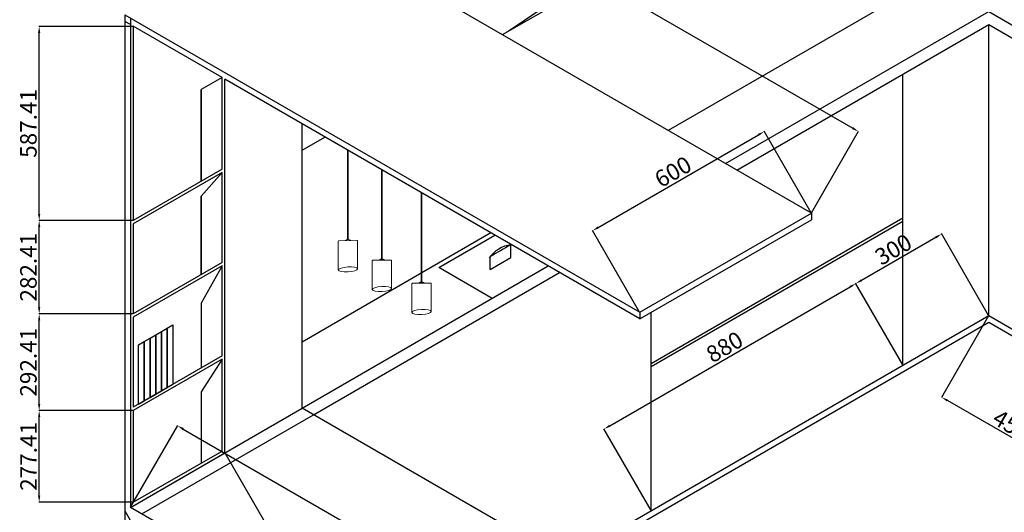
# Model space of a CAD drawing. Units: centimetres. Extents: x 209356 to 217348, y 253987 to 259034.
# Tile 3 of 7: x 209356 to 212337, y 255772 to 257262. Entities that reach past the tile are written whole.
import ezdxf

# ---------------------------------------------------------------- set-up
doc = ezdxf.new("R2010")
doc.units = ezdxf.units.CM
for name, color, linetype, lineweight in [('A-ANNO-DIMS', 2, 'Continuous', 18), ('A-ELEV', 7, 'Continuous', 25), ('E-LITE', 3, 'Continuous', 18)]:
    doc.layers.add(name, color=color, linetype=linetype, lineweight=lineweight)
doc.styles.get("Standard").update_dxf_attribs({"font": 'arial.ttf'})
doc.dimstyles.new('ISO-25', dxfattribs={"dimtxt": 50, "dimasz": 20, "dimexe": 1.25, "dimexo": 0.625, "dimtad": 1, "dimdec": 1, "dimtxsty": 'Standard', "dimcen": 2.5, "dimadec": 0, "dimazin": 0, "dimtfac": 1, "dimtdec": 1, "dimtmove": 0, "dimatfit": 3, "dimfxl": 1, "dimarcsym": 0})

# ---------------------------------------------------------------- blocks, each defined once
blk = doc.blocks.new('LIGHT')
for p, q in [((210344.1, 256869.7), (210344.1, 256599.7)), ((210346.1, 256868.6), (210346.1, 256599.7)), ((210315.9, 256593.8), (210315.9, 256507.2)), ((210317.9, 256595.8), (210372.2, 256596.5)), ((210374.2, 256594.5), (210374.2, 256510.5))]:
    blk.add_line(p, q)
for centre, radius, start, end in [((210345.1, 256588.5), 11.3, 43.6374, 137.8986), ((210317.9, 256593.8), 2, 90.768, 180), ((210345.2, 256587.8), 11.3, 48.5689, 132.9671), ((210372.2, 256594.5), 2, 0, 90.768)]:
    blk.add_arc(centre, radius, start, end)
blk.add_ellipse((210345.1, 256508.8), major_axis=(-29.2, -1.7), ratio=0.258257)
blk = doc.blocks.new('*D12')
at = {"layer": 'A-ANNO-DIMS', "color": 0, "lineweight": -2, "transparency": 16777216}
for p, q in [((209691.8, 255787.1), (209834.6, 256034.4)), ((209851.3, 256023.4), (211375.5, 255143.4)), ((211250.7, 254887.1), (211393.5, 255134.4))]:
    blk.add_line(p, q, dxfattribs=at)
at = {"layer": 'A-ANNO-DIMS', "color": 0, "transparency": 16777216}
for points in [[(209853, 256026.3), (209849.6, 256020.5), (209834, 256033.4)], [(211377.2, 255146.3), (211373.9, 255140.5), (211392.8, 255133.4)]]:
    blk.add_solid(points, dxfattribs=at)
at = {"layer": 'Defpoints', "color": 0, "transparency": 16777216}
for p in [(209691.5, 255786.5), (211392.8, 255133.4), (211250.3, 254886.5)]:
    blk.add_point(p, dxfattribs=at)
at = {"layer": 'A-ANNO-DIMS', "color": 0, "transparency": 16777216, "insert": (210626.5, 255606), "char_height": 50, "attachment_point": 5, "rotation": 330}
blk.add_mtext('1800', dxfattribs=at)
blk = doc.blocks.new('*D15')
at = {"layer": 'A-ANNO-DIMS', "color": 0, "lineweight": -2, "transparency": 16777216}
for p, q in [((212289.3, 256366), (212146.4, 256118.6)), ((212679, 256141), (212536.2, 255893.6)), ((212519.5, 255904.7), (212164.4, 256109.7))]:
    blk.add_line(p, q, dxfattribs=at)
at = {"layer": 'A-ANNO-DIMS', "color": 0, "transparency": 16777216}
for points in [[(212166.1, 256112.6), (212162.7, 256106.8), (212147.1, 256119.7)], [(212521.1, 255907.6), (212517.8, 255901.8), (212536.8, 255894.7)]]:
    blk.add_solid(points, dxfattribs=at)
at = {"layer": 'Defpoints', "color": 0, "transparency": 16777216}
for p in [(212289.6, 256366.5), (212679.3, 256141.5), (212147.1, 256119.7)]:
    blk.add_point(p, dxfattribs=at)
at = {"layer": 'A-ANNO-DIMS', "color": 0, "transparency": 16777216, "insert": (212355, 256029.9), "char_height": 50, "attachment_point": 5, "rotation": 330}
blk.add_mtext('450', dxfattribs=at)
blk = doc.blocks.new('*D30')
at = {"layer": 'A-ANNO-DIMS', "color": 0, "lineweight": -2, "transparency": 16777216}
for p, q in [((209699.5, 256079.3), (209413.9, 256079.3)), ((209415.2, 255821.9), (209415.2, 256059.3)), ((209699.5, 255801.9), (209413.9, 255801.9))]:
    blk.add_line(p, q, dxfattribs=at)
at = {"layer": 'A-ANNO-DIMS', "color": 0, "transparency": 16777216}
for points in [[(209411.8, 256059.3), (209418.5, 256059.3), (209415.2, 256079.3)], [(209411.8, 255821.9), (209418.5, 255821.9), (209415.2, 255801.9)]]:
    blk.add_solid(points, dxfattribs=at)
at = {"layer": 'Defpoints', "color": 0, "transparency": 16777216}
for p in [(209415.2, 256079.3), (209700.2, 256079.3), (209700.2, 255801.9)]:
    blk.add_point(p, dxfattribs=at)
at = {"layer": 'A-ANNO-DIMS', "color": 0, "transparency": 16777216, "insert": (209389.4, 255940.6), "char_height": 50, "attachment_point": 5, "rotation": 90}
blk.add_mtext('277.41', dxfattribs=at)
blk = doc.blocks.new('*D31')
at = {"layer": 'A-ANNO-DIMS', "color": 0, "lineweight": -2, "transparency": 16777216}
for p, q in [((209699.5, 256371.7), (209413.9, 256371.7)), ((209415.2, 256099.3), (209415.2, 256351.7)), ((209699.5, 256079.3), (209413.9, 256079.3))]:
    blk.add_line(p, q, dxfattribs=at)
at = {"layer": 'A-ANNO-DIMS', "color": 0, "transparency": 16777216}
for points in [[(209411.8, 256351.7), (209418.5, 256351.7), (209415.2, 256371.7)], [(209411.8, 256099.3), (209418.5, 256099.3), (209415.2, 256079.3)]]:
    blk.add_solid(points, dxfattribs=at)
at = {"layer": 'Defpoints', "color": 0, "transparency": 16777216}
for p in [(209415.2, 256371.7), (209700.2, 256371.7), (209700.2, 256079.3)]:
    blk.add_point(p, dxfattribs=at)
at = {"layer": 'A-ANNO-DIMS', "color": 0, "transparency": 16777216, "insert": (209389, 256225.5), "char_height": 50, "attachment_point": 5, "rotation": 90}
blk.add_mtext('292.41', dxfattribs=at)
blk = doc.blocks.new('*D32')
at = {"layer": 'A-ANNO-DIMS', "color": 0, "lineweight": -2, "transparency": 16777216}
for p, q in [((209699.5, 256654.1), (209413.9, 256654.1)), ((209415.2, 256391.7), (209415.2, 256634.1)), ((209699.5, 256371.7), (209413.9, 256371.7))]:
    blk.add_line(p, q, dxfattribs=at)
at = {"layer": 'A-ANNO-DIMS', "color": 0, "transparency": 16777216}
for points in [[(209411.8, 256634.1), (209418.5, 256634.1), (209415.2, 256654.1)], [(209411.8, 256391.7), (209418.5, 256391.7), (209415.2, 256371.7)]]:
    blk.add_solid(points, dxfattribs=at)
at = {"layer": 'Defpoints', "color": 0, "transparency": 16777216}
for p in [(209415.2, 256654.1), (209700.2, 256654.1), (209700.2, 256371.7)]:
    blk.add_point(p, dxfattribs=at)
at = {"layer": 'A-ANNO-DIMS', "color": 0, "transparency": 16777216, "insert": (209389, 256512.9), "char_height": 50, "attachment_point": 5, "rotation": 90}
blk.add_mtext('282.41', dxfattribs=at)
blk = doc.blocks.new('*D33')
at = {"layer": 'A-ANNO-DIMS', "color": 0, "lineweight": -2, "transparency": 16777216}
for p, q in [((209699.5, 257241.5), (209413.9, 257241.5)), ((209415.2, 256674.1), (209415.2, 257221.5)), ((209699.5, 256654.1), (209413.9, 256654.1))]:
    blk.add_line(p, q, dxfattribs=at)
at = {"layer": 'A-ANNO-DIMS', "color": 0, "transparency": 16777216}
for points in [[(209411.8, 257221.5), (209418.5, 257221.5), (209415.2, 257241.5)], [(209411.8, 256674.1), (209418.5, 256674.1), (209415.2, 256654.1)]]:
    blk.add_solid(points, dxfattribs=at)
at = {"layer": 'Defpoints', "color": 0, "transparency": 16777216}
for p in [(209415.2, 257241.5), (209700.2, 257241.5), (209700.2, 256654.1)]:
    blk.add_point(p, dxfattribs=at)
at = {"layer": 'A-ANNO-DIMS', "color": 0, "transparency": 16777216, "insert": (209389, 256947.8), "char_height": 50, "attachment_point": 5, "rotation": 90}
blk.add_mtext('587.41', dxfattribs=at)
blk = doc.blocks.new('*D34')
at = {"layer": 'A-ANNO-DIMS', "color": 0, "lineweight": -2, "transparency": 16777216}
for p, q in [((209977.6, 255951), (210120.4, 255703.6)), ((209674.5, 255776), (209817.3, 255528.6)), ((210102.5, 255694.7), (209834, 255539.7))]:
    blk.add_line(p, q, dxfattribs=at)
at = {"layer": 'A-ANNO-DIMS', "color": 0, "transparency": 16777216}
for points in [[(210100.8, 255697.6), (210104.1, 255691.8), (210119.8, 255704.7)], [(209832.3, 255542.6), (209835.7, 255536.8), (209816.7, 255529.7)]]:
    blk.add_solid(points, dxfattribs=at)
at = {"layer": 'Defpoints', "color": 0, "transparency": 16777216}
for p in [(209977.3, 255951.5), (209674.2, 255776.5), (209816.7, 255529.7)]:
    blk.add_point(p, dxfattribs=at)
at = {"layer": 'A-ANNO-DIMS', "color": 0, "transparency": 16777216, "insert": (209955.1, 255639.9), "char_height": 50, "attachment_point": 5, "rotation": 30}
blk.add_mtext('350', dxfattribs=at)
blk = doc.blocks.new('*D35')
at = {"layer": 'A-ANNO-DIMS', "color": 0, "lineweight": -2, "transparency": 16777216}
for p, q in [((210211.4, 257567.1), (210354.2, 257814.4)), ((210370.9, 257803.4), (211877.8, 256933.4)), ((211752.9, 256677.1), (211895.8, 256924.4))]:
    blk.add_line(p, q, dxfattribs=at)
at = {"layer": 'A-ANNO-DIMS', "color": 0, "transparency": 16777216}
for points in [[(210372.6, 257806.3), (210369.3, 257800.5), (210353.6, 257813.4)], [(211879.5, 256936.3), (211876.1, 256930.5), (211895.1, 256923.4)]]:
    blk.add_solid(points, dxfattribs=at)
at = {"layer": 'Defpoints', "color": 0, "transparency": 16777216}
for p in [(210211.1, 257566.5), (211895.1, 256923.4), (211752.6, 256676.5)]:
    blk.add_point(p, dxfattribs=at)
at = {"layer": 'A-ANNO-DIMS', "color": 0, "transparency": 16777216, "insert": (211137.4, 257391), "char_height": 50, "attachment_point": 5, "rotation": 330}
blk.add_mtext('1780', dxfattribs=at)
blk = doc.blocks.new('*D36')
at = {"layer": 'A-ANNO-DIMS', "color": 0, "lineweight": -2, "transparency": 16777216}
for p, q in [((211107.8, 256633.4), (211592.8, 256913.4)), ((211752.3, 256677.1), (211609.5, 256924.4)), ((211232.7, 256377.1), (211089.9, 256624.4))]:
    blk.add_line(p, q, dxfattribs=at)
at = {"layer": 'A-ANNO-DIMS', "color": 0, "transparency": 16777216}
for points in [[(211591.1, 256916.3), (211594.5, 256910.5), (211610.1, 256923.4)], [(211106.2, 256636.3), (211109.5, 256630.5), (211090.5, 256623.4)]]:
    blk.add_solid(points, dxfattribs=at)
at = {"layer": 'Defpoints', "color": 0, "transparency": 16777216}
for p in [(211610.1, 256923.4), (211752.6, 256676.5), (211233, 256376.5)]:
    blk.add_point(p, dxfattribs=at)
at = {"layer": 'A-ANNO-DIMS', "color": 0, "transparency": 16777216, "insert": (211337.2, 256796), "char_height": 50, "attachment_point": 5, "rotation": 30}
blk.add_mtext('600', dxfattribs=at)
blk = doc.blocks.new('*D37')
at = {"layer": 'A-ANNO-DIMS', "color": 0, "lineweight": -2, "transparency": 16777216}
for p, q in [((211142.5, 256033.4), (211869.9, 256453.4)), ((212029.4, 256217.1), (211886.6, 256464.4)), ((211267.3, 255777.1), (211124.5, 256024.4))]:
    blk.add_line(p, q, dxfattribs=at)
at = {"layer": 'A-ANNO-DIMS', "color": 0, "transparency": 16777216}
for points in [[(211868.3, 256456.3), (211871.6, 256450.5), (211887.3, 256463.4)], [(211140.8, 256036.3), (211144.1, 256030.5), (211125.2, 256023.4)]]:
    blk.add_solid(points, dxfattribs=at)
at = {"layer": 'Defpoints', "color": 0, "transparency": 16777216}
for p in [(211887.3, 256463.4), (212029.8, 256216.5), (211267.7, 255776.5)]:
    blk.add_point(p, dxfattribs=at)
at = {"layer": 'A-ANNO-DIMS', "color": 0, "transparency": 16777216, "insert": (211493.1, 256266), "char_height": 50, "attachment_point": 5, "rotation": 30}
blk.add_mtext('880', dxfattribs=at)
blk = doc.blocks.new('*D38')
at = {"layer": 'A-ANNO-DIMS', "color": 0, "lineweight": -2, "transparency": 16777216}
for p, q in [((211904.6, 256473.4), (212129.7, 256603.4)), ((212289.3, 256367.1), (212146.4, 256614.4)), ((212029.4, 256217.1), (211886.6, 256464.4))]:
    blk.add_line(p, q, dxfattribs=at)
at = {"layer": 'A-ANNO-DIMS', "color": 0, "transparency": 16777216}
for points in [[(212128.1, 256606.3), (212131.4, 256600.5), (212147.1, 256613.4)], [(211902.9, 256476.3), (211906.2, 256470.5), (211887.3, 256463.4)]]:
    blk.add_solid(points, dxfattribs=at)
at = {"layer": 'Defpoints', "color": 0, "transparency": 16777216}
for p in [(212147.1, 256613.4), (212289.6, 256366.5), (212029.8, 256216.5)]:
    blk.add_point(p, dxfattribs=at)
at = {"layer": 'A-ANNO-DIMS', "color": 0, "transparency": 16777216, "insert": (212004.1, 256561), "char_height": 50, "attachment_point": 5, "rotation": 30}
blk.add_mtext('300', dxfattribs=at)

msp = doc.modelspace()

# ---------------------------------------------------------------- linework, layer by layer
at = {"layer": 'A-ELEV'}
for p, q in [((210817.3256, 257216.5492), (212289.5688, 258066.5492)), ((211752.633, 256676.5492), (210211.1078, 257566.5492)), ((210834.8943, 257226.6924), (211113.0858, 257415.2401)), ((212186.0099, 257426.7594), (211319.6203, 256926.5492)), ((211492.8254, 256826.5492), (212289.5688, 257286.5492)), ((212289.5688, 257286.5492), (214064.9209, 256261.5492)), ((209674.1721, 257276.5492), (209674.1721, 255776.5492)), ((209674.1721, 257276.5492), (211233.0178, 256376.5492)), ((209691.4926, 257246.5492), (209674.1721, 257256.5492)), ((209691.4926, 257266.5492), (209691.4926, 255786.5492)), ((209700.1528, 257241.5492), (209700.1528, 256654.1374)), ((209968.6207, 257086.5492), (209700.1528, 257241.5492)), ((211527.4664, 256806.5492), (212289.5688, 257246.5492)), ((212289.5688, 257246.5492), (214064.9209, 256221.5492)), ((212289.5688, 256366.5492), (212289.5688, 257246.5492)), ((209968.6207, 257086.5492), (209905.2834, 257049.9813)), ((209968.6207, 256809.1374), (209968.6207, 257086.5492)), ((209977.281, 255951.5492), (209977.281, 257081.5492)), ((211233.0178, 256356.5492), (209977.281, 257081.5492)), ((212029.7612, 256216.5492), (212029.7612, 257096.5492)), ((209905.2834, 257049.9813), (209905.2834, 256772.5696)), ((209905.2834, 256772.5696), (209905.2834, 257049.9813)), ((210211.1078, 256086.5492), (210211.1078, 256946.5492)), ((210211.1078, 256866.5492), (210280.3898, 256906.5492)), ((209968.6207, 256809.1374), (209700.1528, 256654.1374)), ((209968.6207, 256799.1374), (209700.1528, 256644.1374)), ((209968.6207, 256799.1374), (209905.2834, 256727.7953)), ((209968.6207, 256526.7257), (209968.6207, 256799.1374)), ((209905.2834, 256490.1579), (209905.2834, 256727.7953)), ((209905.2834, 256727.7953), (209905.2834, 256490.1579)), ((211233.0178, 256376.5492), (211752.633, 256676.5492)), ((212029.7612, 256661.0964), (211267.6588, 256221.0964)), ((211752.633, 256676.5492), (211752.633, 256656.5492)), ((209700.1528, 256644.1374), (209700.1528, 256371.7257)), ((211233.0178, 256356.5492), (211752.633, 256656.5492)), ((212029.7612, 256651.5492), (211267.6588, 256211.5492)), ((210782.6846, 256616.5492), (210211.1078, 256286.5492)), ((210625.1239, 256511.886), (210794.5452, 256609.7014)), ((210842.7148, 256541.9871), (210842.7148, 256580.6156)), ((210780.5707, 256506.2789), (210780.5707, 256544.9074)), ((210780.5707, 256506.2789), (210842.7148, 256541.9871)), ((209968.6207, 256526.7257), (209700.1528, 256371.7257)), ((209968.6207, 256516.7257), (209700.1528, 256361.7257)), ((209968.6207, 256516.7257), (209905.2834, 256404.493)), ((209968.6207, 256244.314), (209968.6207, 256516.7257)), ((210211.1078, 256086.5492), (210955.8897, 256516.5492)), ((210786.4684, 256418.7337), (210625.1239, 256511.886)), ((210245.7488, 256066.5492), (210990.5307, 256496.5492)), ((209905.2834, 256404.493), (209905.2834, 256207.7462)), ((209700.1528, 256361.7257), (209700.1528, 256089.314)), ((211007.8512, 255626.5492), (212289.5688, 256366.5492)), ((211233.0178, 256376.5492), (211233.0178, 256356.5492)), ((211267.6588, 255776.5492), (211267.6588, 256376.5492)), ((212289.5688, 256366.5492), (214887.645, 254866.5492)), ((209802.7536, 256328.4831), (209820.0741, 256338.4831)), ((209820.0741, 256338.4831), (209820.0741, 256158.5506)), ((211025.1717, 255616.5492), (212289.5688, 256346.5492)), ((212289.5688, 256346.5492), (214887.645, 254846.5492)), ((209750.7921, 256298.4831), (209768.1126, 256308.4831)), ((209768.1126, 256308.4831), (209785.4331, 256318.4831)), ((209768.1126, 256308.4831), (209768.1126, 256128.5506)), ((209768.1126, 256128.5506), (209768.1126, 256308.4831)), ((209785.4331, 256318.4831), (209802.7536, 256328.4831)), ((209785.4331, 256318.4831), (209785.4331, 256138.5506)), ((209785.4331, 256138.5506), (209785.4331, 256318.4831)), ((209802.7536, 256328.4831), (209802.7536, 256148.5506)), ((209802.7536, 256148.5506), (209802.7536, 256328.4831)), ((209716.1511, 256278.4831), (209733.4716, 256288.4831)), ((209716.1511, 256098.5506), (209716.1511, 256278.4831)), ((209733.4716, 256288.4831), (209750.7921, 256298.4831)), ((209733.4716, 256288.4831), (209733.4716, 256108.5506)), ((209733.4716, 256108.5506), (209733.4716, 256288.4831)), ((209750.7921, 256298.4831), (209750.7921, 256118.5506)), ((209750.7921, 256118.5506), (209750.7921, 256298.4831)), ((209968.6207, 256244.314), (209700.1528, 256089.314)), ((209968.6207, 256234.314), (209700.1528, 256079.314)), ((209968.6207, 256234.314), (209905.2834, 256136.0165)), ((209968.6207, 255956.9023), (209968.6207, 256234.314)), ((209802.7536, 256148.5506), (209820.0741, 256158.5506)), ((209750.7921, 256118.5506), (209768.1126, 256128.5506)), ((209768.1126, 256128.5506), (209785.4331, 256138.5506)), ((209785.4331, 256138.5506), (209802.7536, 256148.5506)), ((209905.2834, 256136.0165), (209905.2834, 255920.3345)), ((209716.1511, 256098.5506), (209733.4716, 256108.5506)), ((209733.4716, 256108.5506), (209750.7921, 256118.5506)), ((209691.4926, 255786.5492), (210211.1078, 256086.5492)), ((209700.1528, 256079.314), (209700.1528, 255801.9023)), ((209726.1336, 255766.5492), (210245.7488, 256066.5492)), ((211769.9535, 255186.5492), (210211.1078, 256086.5492)), ((209691.4926, 255786.5492), (209977.281, 255951.5492)), ((209700.1528, 255801.9023), (209968.6207, 255956.9023)), ((209674.1721, 255776.5492), (209674.1721, 254876.5492)), ((211250.3383, 254886.5492), (209691.4926, 255786.5492))]:
    msp.add_line(p, q, dxfattribs=at)
for centre, radius, start, end in [((210855.9241, 256485.6697), 95.8603, 97.474954, 145.0385981), ((215723.0638, 248015.2583), 9858.1515, 119.67352306, 120.09008668)]:
    msp.add_arc(centre, radius, start, end, dxfattribs=at)

# ---------------------------------------------------------------- block references
at = {"layer": 'E-LITE'}
for p in [(4.7165, -2.723), (107.4668, -62.046), (227.5524, -131.3775)]:
    msp.add_blockref('LIGHT', p, dxfattribs=at)

# ---------------------------------------------------------------- dimensions: what is measured, and where the dimension line sits
at = {"layer": 'A-ANNO-DIMS'}
for base, p1, p2, angle, override, picture, middle in [((211895.133, 256923.3664), (210211.1078, 257566.5492), (211752.633, 256676.5492), 330, {"dimdec": 0, "dimlfac": 1, "dimrnd": 0, "dimzin": 0, "dimdsep": 46, "dimlunit": 2}, '*D35', (211137.4472, 257391.0161)), ((209415.1528, 257241.5492), (209700.1528, 256654.1374), (209700.1528, 257241.5492), 90, {"dimdec": 2, "dimlfac": 1, "dimrnd": 0, "dimzin": 0, "dimdsep": 46, "dimlunit": 2}, '*D33', (209388.9992, 256947.8433)), ((211610.133, 256923.3664), (211233.0178, 256376.5492), (211752.633, 256676.5492), 30, {"dimdec": 0, "dimlfac": 1, "dimrnd": 0, "dimzin": 0, "dimdsep": 46, "dimlunit": 2}, '*D36', (211337.2486, 256796.0161)), ((209415.1528, 256654.1374), (209700.1528, 256371.7257), (209700.1528, 256654.1374), 90, {"dimdec": 2, "dimlfac": 1, "dimrnd": 0, "dimzin": 0, "dimdsep": 46, "dimlunit": 2}, '*D32', (209388.9992, 256512.9316)), ((212147.0688, 256613.3664), (212029.7612, 256216.5492), (212289.5688, 256366.5492), 30, {"dimdec": 0, "dimlfac": 1, "dimrnd": 0, "dimzin": 0, "dimdsep": 46, "dimlunit": 2}, '*D38', (212004.0796, 256561.0309)), ((211887.2612, 256463.3664), (211267.6588, 255776.5492), (212029.7612, 256216.5492), 30, {"dimdec": 0, "dimlfac": 1, "dimrnd": 0, "dimzin": 0, "dimdsep": 46, "dimlunit": 2}, '*D37', (211493.1332, 256266.0161)), ((209415.1528, 256371.7257), (209700.1528, 256079.314), (209700.1528, 256371.7257), 90, {"dimdec": 2, "dimlfac": 1, "dimrnd": 0, "dimzin": 0, "dimdsep": 46, "dimlunit": 2}, '*D31', (209388.9992, 256225.5199)), ((212147.0688, 256119.7319), (212679.2802, 256141.5492), (212289.5688, 256366.5492), 150, {"dimdec": 0, "dimlfac": 1, "dimrnd": 0, "dimzin": 0, "dimdsep": 46, "dimlunit": 2}, '*D15', (212355.0013, 256029.8816)), ((209415.1528, 256079.314), (209700.1528, 255801.9023), (209700.1528, 256079.314), 90, {"dimdec": 2, "dimlfac": 1, "dimrnd": 0, "dimzin": 0, "dimdsep": 46, "dimlunit": 2}, '*D30', (209389.4255, 255940.6081)), ((211392.8383, 255133.3664), (209691.4926, 255786.5492), (211250.3383, 254886.5492), 330, {"dimdec": 0, "dimlfac": 1, "dimrnd": 0, "dimzin": 0, "dimdsep": 46, "dimlunit": 2}, '*D12', (210626.4923, 255606.0161)), ((209816.6721, 255529.7319), (209977.281, 255951.5492), (209674.1721, 255776.5492), 210, {"dimdec": 0, "dimlfac": 1, "dimrnd": 0, "dimzin": 0, "dimdsep": 46, "dimlunit": 2}, '*D34', (209955.1412, 255639.8964))]:
    dim = msp.add_linear_dim(base=base, p1=p1, p2=p2, angle=angle, dimstyle='ISO-25', override=override, dxfattribs=at)
    dim.commit()
    dim.dimension.update_dxf_attribs({"geometry": picture, "text_midpoint": middle})

doc.saveas('drawing.dxf')
